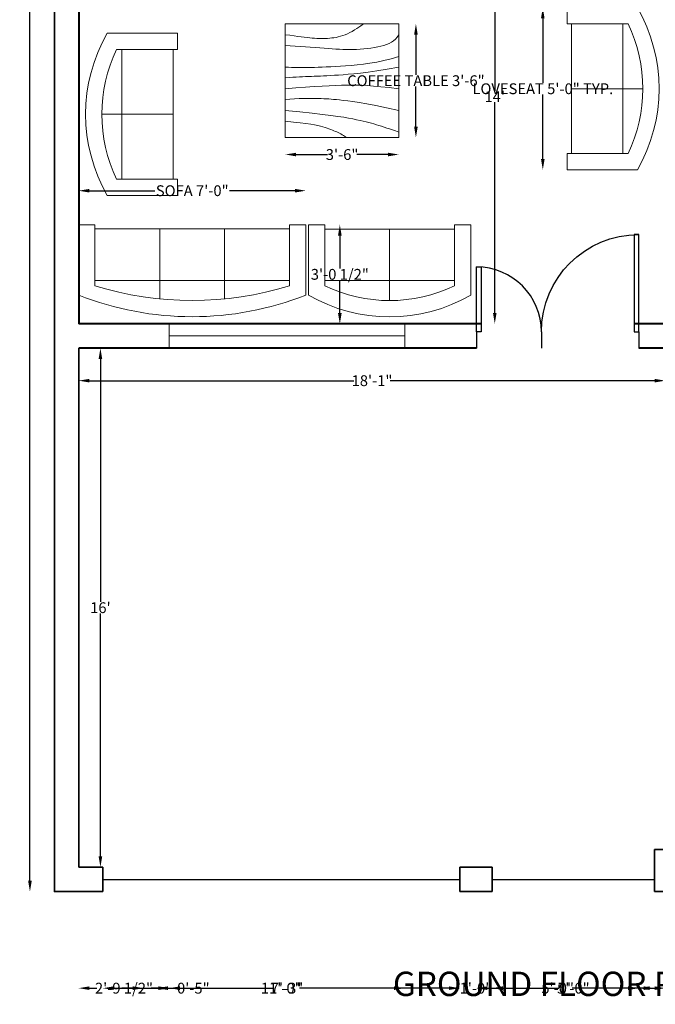
# Model space of a CAD drawing. Units: inches. Extents: x -46 to 447, y -42 to 702.
# Tile 1 of 7: x -13 to 222, y -42 to 322. Entities that reach past the tile are written whole.
import ezdxf

# ---------------------------------------------------------------- set-up
doc = ezdxf.new("R2010")
doc.units = ezdxf.units.IN
doc.header["$PDMODE"] = 3
for name, color, linetype, lineweight in [('A-ANNO-DIMS', 2, 'Continuous', 13), ('A-ANNO-TEXT', 3, 'Continuous', 25), ('A-DOOR', 3, 'Continuous', 25), ('A-FURN', 8, 'Continuous', 18), ('A-GLAZ', 4, 'Continuous', 18), ('A-WALL', 7, 'Continuous', 40), ('L-FENC-GATE', 34, 'Continuous', 25), ('L-WALL', 7, 'Continuous', 35)]:
    doc.layers.add(name, color=color, linetype=linetype, lineweight=lineweight)
doc.styles.get("Standard").update_dxf_attribs({"font": 'arial.ttf'})
doc.dimstyles.get("Standard").update_dxf_attribs({"dimtxt": 4, "dimasz": 4, "dimexe": 0.18, "dimexo": 0.0625, "dimgap": 0.09, "dimtad": 0, "dimtih": 1, "dimtoh": 1, "dimdec": 0, "dimzin": 0, "dimdsep": 46, "dimlunit": 3, "dimtxsty": 'Standard', "dimcen": 0.09, "dimse1": 1, "dimse2": 1, "dimadec": 0, "dimazin": 0, "dimtfac": 1, "dimtdec": 0, "dimtofl": 0, "dimtmove": 0, "dimatfit": 3, "dimfxl": 1, "dimtolj": 1, "dimtzin": 0, "dimarcsym": 0})

# ---------------------------------------------------------------- blocks, each defined once
blk = doc.blocks.new('*U5')
for p, q in [((0, 0), (0, -6)), ((24, 0), (24, -6))]:
    blk.add_line(p, q)
blk.add_lwpolyline([(0, 0), (0, 24), (1.75, 24), (1.75, 0)], close=True)
blk.add_arc((0, 0), 24, 0, 90)
blk = doc.blocks.new('*U6')
for p, q in [((0, 0), (0, -6)), ((36, 0), (36, -6))]:
    blk.add_line(p, q)
blk.add_lwpolyline([(0, 0), (0, 36), (1.75, 36), (1.75, 0)], close=True)
blk.add_arc((0, 0), 36, 0, 90)
blk = doc.blocks.new('Sofa - Roundback Loveseat 5 ft.')
for p, q in [((0, -32.44198), (0, -5.99998)), ((-24, -33.99998), (-24, -11.46958)), ((-23.9998, -13.38178), (23.99986, -13.38178)), ((24.00004, -33.99998), (24.00004, -11.46958)), ((-24, -32.44198), (24.00004, -32.44198))]:
    blk.add_line(p, q)
for points in [[(-24, -33.99998), (-30, -33.99998), (-30, -7.99998)], [(30.00004, -7.99998), (30.00004, -33.99998), (24.00004, -33.99998)]]:
    blk.add_lwpolyline(points)
for centre, radius, start, end in [((0, -60.24998), 60.24998, 60.13715, 119.8628), ((0, -61.38438), 55.38444, 64.32083, 115.6792)]:
    blk.add_arc(centre, radius, start, end)
blk = doc.blocks.new('Sofa - Roundback 7 ft.')
for p, q in [((-12.00002, -32.4421), (-12.00003, -6.5971)), ((11.99997, -32.4421), (11.99998, -6.5971)), ((-36.000027, -34), (-36.000027, -11.4696)), ((-35.999844, -13.3819), (35.9998, -13.3819)), ((35.99998, -34), (35.99998, -11.4696)), ((-36.000027, -32.4421), (35.99998, -32.4421))]:
    blk.add_line(p, q)
for points in [[(-36.000027, -34), (-42.000027, -34), (-42.000027, -8)], [(41.99998, -8), (41.99998, -34), (35.99998, -34)]]:
    blk.add_lwpolyline(points)
for centre, radius, start, end in [((0, -114.25), 114.25, 68.43141, 111.5686), ((-0.00001, -127.1968), 121.1968, 72.72033, 107.2797)]:
    blk.add_arc(centre, radius, start, end)
blk = doc.blocks.new('Table - Square Woodgrain 42 x 42 in.')
blk.add_line((0, -42), (42, -42))
for points in [[(0, -4), (1.704, -4.2172), (3.2358, -4.4188), (4.615, -4.604), (5.8615, -4.7721), (6.9951, -4.9224), (8.0357, -5.0541), (9.0031, -5.1667), (9.9171, -5.2594), (10.7951, -5.3316), (11.6445, -5.3836), (12.4702, -5.4157), (13.277, -5.4283), (14.0698, -5.4217), (14.8535, -5.3964), (15.6331, -5.3526), (16.4133, -5.2908), (17.1986, -5.2103), (17.9913, -5.1062), (18.793, -4.9727), (19.6056, -4.8038), (20.4307, -4.5937), (21.2701, -4.3365), (22.1256, -4.0262), (22.9989, -3.6571), (23.888, -3.2272), (24.7756, -2.7516), (25.6408, -2.2491), (26.4624, -1.7387), (27.2195, -1.2395), (27.891, -0.7703), (28.456, -0.3501), (28.8934, 0.002)], [(0, -42), (0, 0), (42, 0), (42, -42)], [(0, -8), (1.8203, -8.1001), (3.6741, -8.2149), (5.5411, -8.3408), (7.4011, -8.4741), (9.2339, -8.6112), (11.0193, -8.7484), (12.7371, -8.8821), (14.3671, -9.0086), (15.8954, -9.1246), (17.3337, -9.2278), (18.6997, -9.3159), (20.0116, -9.387), (21.2871, -9.4389), (22.5442, -9.4696), (23.8008, -9.477), (25.0749, -9.459), (26.3791, -9.4137), (27.7049, -9.3403), (29.0383, -9.2382), (30.3655, -9.1068), (31.6728, -8.9455), (32.9461, -8.7535), (34.1717, -8.5304), (35.3358, -8.2756), (36.4268, -7.9863), (37.443, -7.6521), (38.3849, -7.2603), (39.253, -6.7986), (40.048, -6.2542), (40.7705, -5.6147), (41.421, -4.8674), (42, -4)], [(42, -12), (39.1784, -12.8621), (36.4519, -13.5654), (33.8246, -14.1294), (31.3004, -14.5731), (28.8832, -14.9161), (26.577, -15.1775), (24.3858, -15.3768), (22.3136, -15.5332), (20.3622, -15.6632), (18.5254, -15.7718), (16.7947, -15.8612), (15.1618, -15.9338), (13.6183, -15.9916), (12.1558, -16.0369), (10.7659, -16.0718), (9.4403, -16.0987), (8.1703, -16.1191), (6.9461, -16.1325), (5.7577, -16.1377), (4.595, -16.1335), (3.4479, -16.1188), (2.3064, -16.0924), (1.1604, -16.0532), (0, -16)], [(42, -16), (37.6529, -16.7365), (33.8802, -17.329), (30.6179, -17.7961), (27.8015, -18.1561), (25.3668, -18.4275), (23.2497, -18.6288), (21.3859, -18.7785), (19.7111, -18.8949), (18.1693, -18.9939), (16.7375, -19.0795), (15.401, -19.1534), (14.1449, -19.217), (12.9544, -19.2717), (11.8148, -19.3191), (10.7113, -19.3606), (9.6291, -19.3976), (8.5534, -19.4323), (7.47, -19.4689), (6.3643, -19.5122), (5.222, -19.5672), (4.0288, -19.6386), (2.7703, -19.7313), (1.4321, -19.8501), (0, -20)], [(0, -24), (3.9243, -23.6805), (7.4766, -23.4138), (10.6891, -23.1954), (13.5943, -23.0205), (16.2247, -22.8847), (18.6125, -22.7832), (20.7903, -22.7116), (22.7903, -22.6651), (24.6563, -22.642), (26.4764, -22.6507), (28.35, -22.7024), (30.3766, -22.8084), (32.6555, -22.98), (35.2861, -23.2283), (38.3678, -23.5645), (42, -24)], [(42, -32), (37.392, -31.017), (33.4585, -30.2231), (30.1291, -29.5949), (27.3334, -29.109), (25.0009, -28.742), (23.0612, -28.4707), (21.4439, -28.2716), (20.0786, -28.1215), (18.8998, -28.0002), (17.8609, -27.9014), (16.9206, -27.8219), (16.0371, -27.7588), (15.1691, -27.709), (14.2748, -27.6693), (13.3128, -27.6368), (12.2415, -27.6083), (11.0295, -27.5824), (9.6867, -27.5643), (8.233, -27.5608), (6.6884, -27.5787), (5.0728, -27.6248), (3.4062, -27.7058), (1.7086, -27.8286), (0, -28)], [(0, -32), (5.4026, -32.5358), (9.9494, -33.019), (13.7424, -33.4553), (16.8834, -33.8505), (19.4743, -34.2106), (21.6171, -34.5413), (23.4136, -34.8486), (24.9657, -35.1382), (26.3614, -35.4156), (27.6332, -35.6841), (28.7995, -35.9467), (29.8788, -36.2064), (30.8897, -36.4661), (31.8507, -36.7288), (32.7802, -36.9973), (33.6968, -37.2747), (34.6175, -37.5635), (35.5531, -37.8651), (36.5128, -38.1805), (37.506, -38.5108), (38.5421, -38.8568), (39.6302, -39.2197), (40.7797, -39.6004), (42, -40)], [(0, -36), (3.0098, -36.2857), (5.5354, -36.5643), (7.6368, -36.8359), (9.374, -37.1009), (10.807, -37.3597), (11.9957, -37.6126), (13.0002, -37.8599), (13.8804, -38.102), (14.6874, -38.3393), (15.4365, -38.5729), (16.1338, -38.8041), (16.7858, -39.0341), (17.3987, -39.264), (17.9787, -39.4952), (18.5322, -39.7288), (19.0655, -39.9662), (19.5832, -40.2081), (20.0842, -40.4544), (20.5657, -40.7046), (21.0249, -40.9581), (21.459, -41.2144), (21.8653, -41.4731), (22.2409, -41.7335), (22.5831, -41.9951)]]:
    blk.add_lwpolyline(points)
blk = doc.blocks.new('*D50')
at = {"layer": 'A-ANNO-DIMS', "color": 0, "lineweight": -2, "transparency": 16777216}
for p, q in [((-9.03, 656), (-9.03, 332.12)), ((-9.03, 4), (-9.03, 327.88))]:
    blk.add_line(p, q, dxfattribs=at)
at = {"layer": 'A-ANNO-DIMS', "color": 0, "transparency": 16777216}
for points in [[(-9.7, 656), (-8.36, 656), (-9.03, 660)], [(-9.7, 4), (-8.36, 4), (-9.03, 0)]]:
    blk.add_solid(points, dxfattribs=at)
at = {"layer": 'Defpoints', "color": 0, "transparency": 16777216}
for p in [(0, 660), (0, 0), (-9.03, 0)]:
    blk.add_point(p, dxfattribs=at)
at = {"layer": 'A-ANNO-DIMS', "color": 0, "transparency": 16777216, "insert": (-9.03, 330), "char_height": 4, "attachment_point": 5}
blk.add_mtext("\\A1;55'", dxfattribs=at)
blk = doc.blocks.new('*D51')
at = {"layer": 'A-ANNO-DIMS', "color": 0, "lineweight": -2, "transparency": 16777216}
for p, q in [((17.04, 197), (17.04, 107.13)), ((17.04, 13), (17.04, 102.87))]:
    blk.add_line(p, q, dxfattribs=at)
at = {"layer": 'A-ANNO-DIMS', "color": 0, "transparency": 16777216}
for points in [[(16.38, 197), (17.71, 197), (17.04, 201)], [(16.38, 13), (17.71, 13), (17.04, 9)]]:
    blk.add_solid(points, dxfattribs=at)
at = {"layer": 'Defpoints', "color": 0, "transparency": 16777216}
for p in [(9, 201), (9, 9), (17.04, 9)]:
    blk.add_point(p, dxfattribs=at)
at = {"layer": 'A-ANNO-DIMS', "color": 0, "transparency": 16777216, "insert": (17.04, 105), "char_height": 4, "attachment_point": 5}
blk.add_mtext("\\A1;16'", dxfattribs=at)
blk = doc.blocks.new('*D52')
at = {"layer": 'A-ANNO-DIMS', "color": 0, "lineweight": -2, "transparency": 16777216}
for p, q in [((13, 188.95), (110.73, 188.95)), ((222, 188.95), (124.27, 188.95))]:
    blk.add_line(p, q, dxfattribs=at)
at = {"layer": 'A-ANNO-DIMS', "color": 0, "transparency": 16777216}
for points in [[(13, 189.62), (13, 188.29), (9, 188.95)], [(222, 189.62), (222, 188.29), (226, 188.95)]]:
    blk.add_solid(points, dxfattribs=at)
at = {"layer": 'Defpoints', "color": 0, "transparency": 16777216}
for p in [(226, 188.95), (9, 180.86), (226, 180.86)]:
    blk.add_point(p, dxfattribs=at)
at = {"layer": 'A-ANNO-DIMS', "color": 0, "transparency": 16777216, "insert": (117.5, 188.95), "char_height": 4, "attachment_point": 5}
blk.add_mtext('\\A1;18\'-1"', dxfattribs=at)
blk = doc.blocks.new('*D64')
at = {"layer": 'A-ANNO-DIMS', "color": 0, "lineweight": -2, "transparency": 16777216}
for p, q in [((162.92, 374), (162.92, 296.1)), ((162.92, 214), (162.92, 291.9))]:
    blk.add_line(p, q, dxfattribs=at)
at = {"layer": 'A-ANNO-DIMS', "color": 0, "transparency": 16777216}
for points in [[(162.25, 374), (163.58, 374), (162.92, 378)], [(162.25, 214), (163.58, 214), (162.92, 210)]]:
    blk.add_solid(points, dxfattribs=at)
at = {"layer": 'Defpoints', "color": 0, "transparency": 16777216}
for p in [(9, 378), (9, 210), (162.92, 210)]:
    blk.add_point(p, dxfattribs=at)
at = {"layer": 'A-ANNO-DIMS', "color": 0, "transparency": 16777216, "insert": (162.92, 294), "char_height": 4, "attachment_point": 5}
blk.add_mtext("\\A1;14'", dxfattribs=at)
blk = doc.blocks.new('*D106')
at = {"layer": 'A-ANNO-DIMS', "color": 0, "lineweight": -2, "transparency": 16777216}
for p, q in [((180.68, 322.9), (180.68, 299.06)), ((180.68, 270.9), (180.68, 294.74))]:
    blk.add_line(p, q, dxfattribs=at)
at = {"layer": 'A-ANNO-DIMS', "color": 0, "transparency": 16777216}
for points in [[(180.01, 322.9), (181.34, 322.9), (180.68, 326.9)], [(180.01, 270.9), (181.34, 270.9), (180.68, 266.9)]]:
    blk.add_solid(points, dxfattribs=at)
at = {"layer": 'Defpoints', "color": 0, "transparency": 16777216}
for p in [(180.68, 326.9), (189.68, 326.9), (189.68, 266.9)]:
    blk.add_point(p, dxfattribs=at)
at = {"layer": 'A-ANNO-DIMS', "color": 0, "transparency": 16777216, "insert": (180.68, 296.9), "char_height": 4, "attachment_point": 5}
blk.add_mtext('\\A1;LOVESEAT 5\'-0" TYP.', dxfattribs=at)
blk = doc.blocks.new('*D108')
at = {"layer": 'A-ANNO-DIMS', "color": 0, "lineweight": -2, "transparency": 16777216}
for p, q in [((13, 259.2), (37.22, 259.2)), ((89, 259.2), (64.78, 259.2))]:
    blk.add_line(p, q, dxfattribs=at)
at = {"layer": 'A-ANNO-DIMS', "color": 0, "transparency": 16777216}
for points in [[(13, 259.87), (13, 258.53), (9, 259.2)], [(89, 259.87), (89, 258.53), (93, 259.2)]]:
    blk.add_solid(points, dxfattribs=at)
at = {"layer": 'Defpoints', "color": 0, "transparency": 16777216}
for p in [(93, 259.2), (9, 246.6), (93, 246.6)]:
    blk.add_point(p, dxfattribs=at)
at = {"layer": 'A-ANNO-DIMS', "color": 0, "transparency": 16777216, "insert": (51, 259.2), "char_height": 4, "attachment_point": 5}
blk.add_mtext('\\A1;SOFA 7\'-0"', dxfattribs=at)
blk = doc.blocks.new('*D109')
at = {"layer": 'A-ANNO-DIMS', "color": 0, "lineweight": -2, "transparency": 16777216}
for p, q in [((105.6, 242.6), (105.6, 230.43)), ((105.6, 213.93), (105.6, 226.11))]:
    blk.add_line(p, q, dxfattribs=at)
at = {"layer": 'A-ANNO-DIMS', "color": 0, "transparency": 16777216}
for points in [[(104.93, 242.6), (106.27, 242.6), (105.6, 246.6)], [(104.93, 213.93), (106.27, 213.93), (105.6, 209.93)]]:
    blk.add_solid(points, dxfattribs=at)
at = {"layer": 'Defpoints', "color": 0, "transparency": 16777216}
for p in [(93, 246.6), (93, 209.93), (105.6, 209.93)]:
    blk.add_point(p, dxfattribs=at)
at = {"layer": 'A-ANNO-DIMS', "color": 0, "transparency": 16777216, "insert": (105.6, 228.27), "char_height": 4, "attachment_point": 5}
blk.add_mtext('\\A1;3\'-0 1/2"', dxfattribs=at)
blk = doc.blocks.new('*D110')
at = {"layer": 'A-ANNO-DIMS', "color": 0, "lineweight": -2, "transparency": 16777216}
for p, q in [((133.74, 316.88), (133.74, 302.04)), ((133.74, 282.88), (133.74, 297.72))]:
    blk.add_line(p, q, dxfattribs=at)
at = {"layer": 'A-ANNO-DIMS', "color": 0, "transparency": 16777216}
for points in [[(133.07, 316.88), (134.41, 316.88), (133.74, 320.88)], [(133.07, 282.88), (134.41, 282.88), (133.74, 278.88)]]:
    blk.add_solid(points, dxfattribs=at)
at = {"layer": 'Defpoints', "color": 0, "transparency": 16777216}
for p in [(127.44, 320.88), (133.74, 320.88), (127.44, 278.88)]:
    blk.add_point(p, dxfattribs=at)
at = {"layer": 'A-ANNO-DIMS', "color": 0, "transparency": 16777216, "insert": (133.74, 299.88), "char_height": 4, "attachment_point": 5}
blk.add_mtext('\\A1;COFFEE TABLE 3\'-6"', dxfattribs=at)
blk = doc.blocks.new('*D111')
at = {"layer": 'A-ANNO-DIMS', "color": 0, "lineweight": -2, "transparency": 16777216}
for p, q in [((89.44, 272.58), (101.04, 272.58)), ((123.44, 272.58), (111.85, 272.58))]:
    blk.add_line(p, q, dxfattribs=at)
at = {"layer": 'A-ANNO-DIMS', "color": 0, "transparency": 16777216}
for points in [[(89.44, 273.24), (89.44, 271.91), (85.44, 272.58)], [(123.44, 273.24), (123.44, 271.91), (127.44, 272.58)]]:
    blk.add_solid(points, dxfattribs=at)
at = {"layer": 'Defpoints', "color": 0, "transparency": 16777216}
for p in [(85.44, 278.88), (127.44, 278.88), (127.44, 272.58)]:
    blk.add_point(p, dxfattribs=at)
at = {"layer": 'A-ANNO-DIMS', "color": 0, "transparency": 16777216, "insert": (106.44, 272.58), "char_height": 4, "attachment_point": 5}
blk.add_mtext('\\A1;3\'-6"', dxfattribs=at)
blk = doc.blocks.new('*D121')
at = {"layer": 'A-ANNO-DIMS', "color": 0, "lineweight": -2, "transparency": 16777216}
for p, q in [((160.17, -35.7), (180.77, -35.7)), ((212.17, -35.7), (191.58, -35.7))]:
    blk.add_line(p, q, dxfattribs=at)
at = {"layer": 'A-ANNO-DIMS', "color": 0, "transparency": 16777216}
for points in [[(160.17, -35.03), (160.17, -36.37), (156.17, -35.7)], [(212.17, -35.03), (212.17, -36.37), (216.17, -35.7)]]:
    blk.add_solid(points, dxfattribs=at)
at = {"layer": 'Defpoints', "color": 0, "transparency": 16777216}
for p in [(156.17, 201), (216.17, 201), (216.17, -35.7)]:
    blk.add_point(p, dxfattribs=at)
at = {"layer": 'A-ANNO-DIMS', "color": 0, "transparency": 16777216, "insert": (186.17, -35.7), "char_height": 4, "attachment_point": 5}
blk.add_mtext('\\A1;5\'-0"', dxfattribs=at)
blk = doc.blocks.new('*D122')
at = {"layer": 'A-ANNO-DIMS', "color": 0, "lineweight": -2, "transparency": 16777216}
for p, q in [((46.51, -35.7), (80.67, -35.7)), ((125.61, -35.7), (91.45, -35.7))]:
    blk.add_line(p, q, dxfattribs=at)
at = {"layer": 'A-ANNO-DIMS', "color": 0, "transparency": 16777216}
for points in [[(46.51, -35.03), (46.51, -36.37), (42.51, -35.7)], [(125.61, -35.03), (125.61, -36.37), (129.61, -35.7)]]:
    blk.add_solid(points, dxfattribs=at)
at = {"layer": 'Defpoints', "color": 0, "transparency": 16777216}
for p in [(42.51, 201), (129.61, 201), (129.61, -35.7)]:
    blk.add_point(p, dxfattribs=at)
at = {"layer": 'A-ANNO-DIMS', "color": 0, "transparency": 16777216, "insert": (86.06, -35.7), "char_height": 4, "attachment_point": 5}
blk.add_mtext('\\A1;7\'-3"', dxfattribs=at)
blk = doc.blocks.new('*D123')
at = {"layer": 'A-ANNO-DIMS', "color": 0, "lineweight": -2, "transparency": 16777216}
for p, q in [((13, -35.7), (15.66, -35.7)), ((38.51, -35.7), (35.86, -35.7))]:
    blk.add_line(p, q, dxfattribs=at)
at = {"layer": 'A-ANNO-DIMS', "color": 0, "transparency": 16777216}
for points in [[(13, -35.03), (13, -36.37), (9, -35.7)], [(38.51, -35.03), (38.51, -36.37), (42.51, -35.7)]]:
    blk.add_solid(points, dxfattribs=at)
at = {"layer": 'Defpoints', "color": 0, "transparency": 16777216}
for p in [(9, 201), (42.51, 201), (42.51, -35.7)]:
    blk.add_point(p, dxfattribs=at)
at = {"layer": 'A-ANNO-DIMS', "color": 0, "transparency": 16777216, "insert": (25.76, -35.7), "char_height": 4, "attachment_point": 5}
blk.add_mtext('\\A1;2\'-9 1/2"', dxfattribs=at)
blk = doc.blocks.new('*D129')
at = {"layer": 'A-ANNO-DIMS', "color": 0, "lineweight": -2, "transparency": 16777216}
for p, q in [((29, -35.7), (25, -35.7)), ((42, -35.7), (46, -35.7))]:
    blk.add_line(p, q, dxfattribs=at)
at = {"layer": 'A-ANNO-DIMS', "color": 0, "transparency": 16777216}
for points in [[(29, -35.03), (29, -36.37), (33, -35.7)], [(42, -35.03), (42, -36.37), (38, -35.7)]]:
    blk.add_solid(points, dxfattribs=at)
at = {"layer": 'Defpoints', "color": 0, "transparency": 16777216}
for p in [(33, 383), (38, 383), (38, -35.7)]:
    blk.add_point(p, dxfattribs=at)
at = {"layer": 'A-ANNO-DIMS', "color": 0, "transparency": 16777216, "insert": (51.41, -35.7), "char_height": 4, "attachment_point": 5}
blk.add_mtext('\\A1;0\'-5"', dxfattribs=at)
blk = doc.blocks.new('*D143')
at = {"layer": 'A-ANNO-DIMS', "color": 0, "lineweight": -2, "transparency": 16777216}
for p, q in [((220.17, -35.7), (222, -35.7)), ((226, -35.7), (230, -35.7))]:
    blk.add_line(p, q, dxfattribs=at)
at = {"layer": 'A-ANNO-DIMS', "color": 0, "transparency": 16777216}
for points in [[(220.17, -35.03), (220.17, -36.37), (216.17, -35.7)], [(222, -35.03), (222, -36.37), (226, -35.7)]]:
    blk.add_solid(points, dxfattribs=at)
at = {"layer": 'Defpoints', "color": 0, "transparency": 16777216}
for p in [(216.17, 201), (226, 201), (226, -35.7)]:
    blk.add_point(p, dxfattribs=at)
at = {"layer": 'A-ANNO-DIMS', "color": 0, "transparency": 16777216, "insert": (236.96, -35.7), "char_height": 4, "attachment_point": 5}
blk.add_mtext('\\A1;0\'-10"', dxfattribs=at)
blk = doc.blocks.new('*D144')
at = {"layer": 'A-ANNO-DIMS', "color": 0, "lineweight": -2, "transparency": 16777216}
for p, q in [((21.93, -35.7), (77.16, -35.7)), ((145.93, -35.7), (90.7, -35.7))]:
    blk.add_line(p, q, dxfattribs=at)
at = {"layer": 'A-ANNO-DIMS', "color": 0, "transparency": 16777216}
for points in [[(21.93, -35.03), (21.93, -36.37), (17.93, -35.7)], [(145.93, -35.03), (145.93, -36.37), (149.93, -35.7)]]:
    blk.add_solid(points, dxfattribs=at)
at = {"layer": 'Defpoints', "color": 0, "transparency": 16777216}
for p in [(17.93, 9), (149.93, 9), (149.93, -35.7)]:
    blk.add_point(p, dxfattribs=at)
at = {"layer": 'A-ANNO-DIMS', "color": 0, "transparency": 16777216, "insert": (83.93, -35.7), "char_height": 4, "attachment_point": 5}
blk.add_mtext('\\A1;11\'-0"', dxfattribs=at)
blk = doc.blocks.new('*D145')
at = {"layer": 'A-ANNO-DIMS', "color": 0, "lineweight": -2, "transparency": 16777216}
for p, q in [((145.93, -35.7), (141.93, -35.7)), ((165.93, -35.7), (169.93, -35.7))]:
    blk.add_line(p, q, dxfattribs=at)
at = {"layer": 'A-ANNO-DIMS', "color": 0, "transparency": 16777216}
for points in [[(145.93, -35.03), (145.93, -36.37), (149.93, -35.7)], [(165.93, -35.03), (165.93, -36.37), (161.93, -35.7)]]:
    blk.add_solid(points, dxfattribs=at)
at = {"layer": 'Defpoints', "color": 0, "transparency": 16777216}
for p in [(149.93, 9), (161.93, 9), (161.93, -35.7)]:
    blk.add_point(p, dxfattribs=at)
at = {"layer": 'A-ANNO-DIMS', "color": 0, "transparency": 16777216, "insert": (155.93, -35.7), "char_height": 4, "attachment_point": 5}
blk.add_mtext('\\A1;1\'-0"', dxfattribs=at)
blk = doc.blocks.new('*D146')
at = {"layer": 'A-ANNO-DIMS', "color": 0, "lineweight": -2, "transparency": 16777216}
for p, q in [((165.93, -35.7), (186.56, -35.7)), ((218, -35.7), (197.37, -35.7))]:
    blk.add_line(p, q, dxfattribs=at)
at = {"layer": 'A-ANNO-DIMS', "color": 0, "transparency": 16777216}
for points in [[(165.93, -35.03), (165.93, -36.37), (161.93, -35.7)], [(218, -35.03), (218, -36.37), (222, -35.7)]]:
    blk.add_solid(points, dxfattribs=at)
at = {"layer": 'Defpoints', "color": 0, "transparency": 16777216}
for p in [(222, 15.54), (161.93, 9), (222, -35.7)]:
    blk.add_point(p, dxfattribs=at)
at = {"layer": 'A-ANNO-DIMS', "color": 0, "transparency": 16777216, "insert": (191.97, -35.7), "char_height": 4, "attachment_point": 5}
blk.add_mtext('\\A1;5\'-0"', dxfattribs=at)

msp = doc.modelspace()

# ---------------------------------------------------------------- linework, layer by layer
at = {"layer": 'A-GLAZ'}
for p, q in [((42.51, 210), (42.51, 201)), ((129.61, 210), (129.61, 201)), ((42.51, 205.5), (129.61, 205.5))]:
    msp.add_line(p, q, dxfattribs=at)
at = {"layer": 'A-WALL'}
for p, q in [((9, 378), (9, 210)), ((157.92, 210), (9, 210)), ((180.3, 210), (179.99, 210)), ((226, 210), (214.42, 210)), ((156.17, 201), (9, 201)), ((226, 201), (216.17, 201))]:
    msp.add_line(p, q, dxfattribs=at)
at = {"layer": 'L-FENC-GATE'}
for p, q in [((17.93, 4.5), (149.93, 4.5)), ((161.93, 4.5), (222, 4.5))]:
    msp.add_line(p, q, dxfattribs=at)
at = {"layer": 'L-WALL'}
for p, q in [((9, 201), (9, 9)), ((222, 15.54), (222, 0)), ((231, 15.54), (222, 15.54)), ((9, 9), (17.93, 9)), ((17.93, 9), (17.93, 0)), ((149.93, 9), (149.93, 0)), ((149.93, 9), (161.93, 9)), ((161.93, 9), (161.93, 0))]:
    msp.add_line(p, q, dxfattribs=at)
for points in [[(222, 0), (396, 0), (396, 660), (0, 660), (0, 0), (17.93, 0)], [(149.93, 0), (161.93, 0)]]:
    msp.add_lwpolyline(points, dxfattribs=at)

# ---------------------------------------------------------------- block references
at = {"layer": 'A-DOOR', "xscale": -1}
msp.add_blockref('*U6', (216.17, 207), dxfattribs=at)
at = {"layer": 'A-DOOR'}
msp.add_blockref('*U5', (156.17, 207), dxfattribs=at)
at = {"layer": 'A-FURN', "xscale": -1}
for name, p, rotation in [('Sofa - Roundback Loveseat 5 ft.', (223.68, 296.9), 270), ('Sofa - Roundback Loveseat 5 ft.', (11.56, 287.47), 90), ('Sofa - Roundback 7 ft.', (51, 212.6), 180), ('Sofa - Roundback Loveseat 5 ft.', (124.03, 212.57), 180)]:
    msp.add_blockref(name, p, dxfattribs=dict(at, rotation=rotation))
at = {"layer": 'A-FURN'}
msp.add_blockref('Table - Square Woodgrain 42 x 42 in.', (85.44, 320.88), dxfattribs=at)

# ---------------------------------------------------------------- texts
at = {"layer": 'A-ANNO-TEXT', "insert": (125.24, -29.6), "char_height": 9, "attachment_point": 1}
msp.add_mtext_dynamic_manual_height_columns('GROUND FLOOR PLAN', width=170.7105, gutter_width=12.5, heights=[0], dxfattribs=at)

# ---------------------------------------------------------------- dimensions: what is measured, and where the dimension line sits
at = {"layer": 'A-ANNO-DIMS'}
for base, p1, p2, angle, override, picture, middle in [((-9.03, 0), (0, 660), (0, 0), 90, {"dimclrd": 0, "dimclre": 0, "dimclrt": 0}, '*D50', (-9.03, 330)), ((162.92, 210), (9, 378), (9, 210), 90, {"dimclrd": 0, "dimclre": 0, "dimclrt": 0}, '*D64', (162.92, 294)), ((105.6, 209.93), (93, 246.6), (93, 209.93), 270, {"dimdec": 1, "dimlfac": 1, "dimrnd": 0, "dimzin": 1, "dimdsep": 46, "dimlunit": 4, "dimfrac": 2}, '*D109', (105.6, 228.27)), ((17.04, 9), (9, 201), (9, 9), 90, {"dimclrd": 0, "dimclre": 0, "dimclrt": 0}, '*D51', (17.04, 105))]:
    dim = msp.add_linear_dim(base=base, p1=p1, p2=p2, angle=angle, dimstyle='Standard', override=override, dxfattribs=at)
    dim.commit()
    dim.dimension.update_dxf_attribs({"geometry": picture, "text_midpoint": middle})
for base, p1, p2, override, picture, middle in [((38, -35.7), (33, 383), (38, 383), {"dimdec": 1, "dimlfac": 1, "dimrnd": 0, "dimzin": 1, "dimdsep": 46, "dimlunit": 4, "dimfrac": 2}, '*D129', (51.41, -35.7)), ((127.44, 272.58), (85.44, 278.88), (127.44, 278.88), {"dimdec": 1, "dimlfac": 1, "dimrnd": 0, "dimzin": 1, "dimdsep": 46, "dimlunit": 4, "dimfrac": 2}, '*D111', (106.44, 272.58)), ((42.51, -35.7), (9, 201), (42.51, 201), {"dimdec": 1, "dimlfac": 1, "dimrnd": 0, "dimzin": 1, "dimdsep": 46, "dimlunit": 4, "dimfrac": 2}, '*D123', (25.76, -35.7)), ((129.61, -35.7), (42.51, 201), (129.61, 201), {"dimdec": 1, "dimlfac": 1, "dimrnd": 0, "dimzin": 1, "dimdsep": 46, "dimlunit": 4, "dimfrac": 2}, '*D122', (86.06, -35.7)), ((216.17, -35.7), (156.17, 201), (216.17, 201), {"dimdec": 1, "dimlfac": 1, "dimrnd": 0, "dimzin": 1, "dimdsep": 46, "dimlunit": 4, "dimfrac": 2}, '*D121', (186.17, -35.7)), ((226, -35.7), (216.17, 201), (226, 201), {"dimdec": 1, "dimlfac": 1, "dimrnd": 0, "dimzin": 1, "dimdsep": 46, "dimlunit": 4, "dimfrac": 2}, '*D143', (236.96, -35.7)), ((226, 188.95), (9, 180.86), (226, 180.86), {"dimclrd": 0, "dimclre": 0, "dimclrt": 0}, '*D52', (117.5, 188.95)), ((222, -35.7), (161.93, 9), (222, 15.54), {"dimdec": 1, "dimlfac": 1, "dimrnd": 0, "dimzin": 1, "dimdsep": 46, "dimlunit": 4, "dimfrac": 2}, '*D146', (191.97, -35.7)), ((149.93, -35.7), (17.93, 9), (149.93, 9), {"dimdec": 1, "dimlfac": 1, "dimrnd": 0, "dimzin": 1, "dimdsep": 46, "dimlunit": 4, "dimfrac": 2}, '*D144', (83.93, -35.7)), ((161.93, -35.7), (149.93, 9), (161.93, 9), {"dimdec": 1, "dimlfac": 1, "dimrnd": 0, "dimzin": 1, "dimdsep": 46, "dimlunit": 4, "dimfrac": 2}, '*D145', (155.93, -35.7))]:
    dim = msp.add_linear_dim(base=base, p1=p1, p2=p2, dimstyle='Standard', override=override, dxfattribs=at)
    dim.commit()
    dim.dimension.update_dxf_attribs({"geometry": picture, "text_midpoint": middle})
for base, p1, p2, text, picture, middle in [((180.68, 326.9), (189.68, 266.9), (189.68, 326.9), 'LOVESEAT <> TYP.', '*D106', (180.68, 296.9)), ((133.74, 320.88), (127.44, 278.88), (127.44, 320.88), 'COFFEE TABLE <>', '*D110', (133.74, 299.88))]:
    dim = msp.add_linear_dim(base=base, p1=p1, p2=p2, angle=90, text=text, dimstyle='Standard', override={"dimdec": 1, "dimlfac": 1, "dimrnd": 0, "dimzin": 1, "dimdsep": 46, "dimlunit": 4, "dimfrac": 2}, dxfattribs=at)
    dim.commit()
    dim.dimension.update_dxf_attribs({"geometry": picture, "text_midpoint": middle})
dim = msp.add_linear_dim(base=(93, 259.2), p1=(9, 246.6), p2=(93, 246.6), text='SOFA <>', dimstyle='Standard', override={"dimdec": 1, "dimlfac": 1, "dimrnd": 0, "dimzin": 1, "dimdsep": 46, "dimlunit": 4, "dimfrac": 2}, dxfattribs=at)
dim.commit()
dim.dimension.update_dxf_attribs({"geometry": '*D108', "text_midpoint": (51, 259.2)})

doc.saveas('drawing.dxf')
